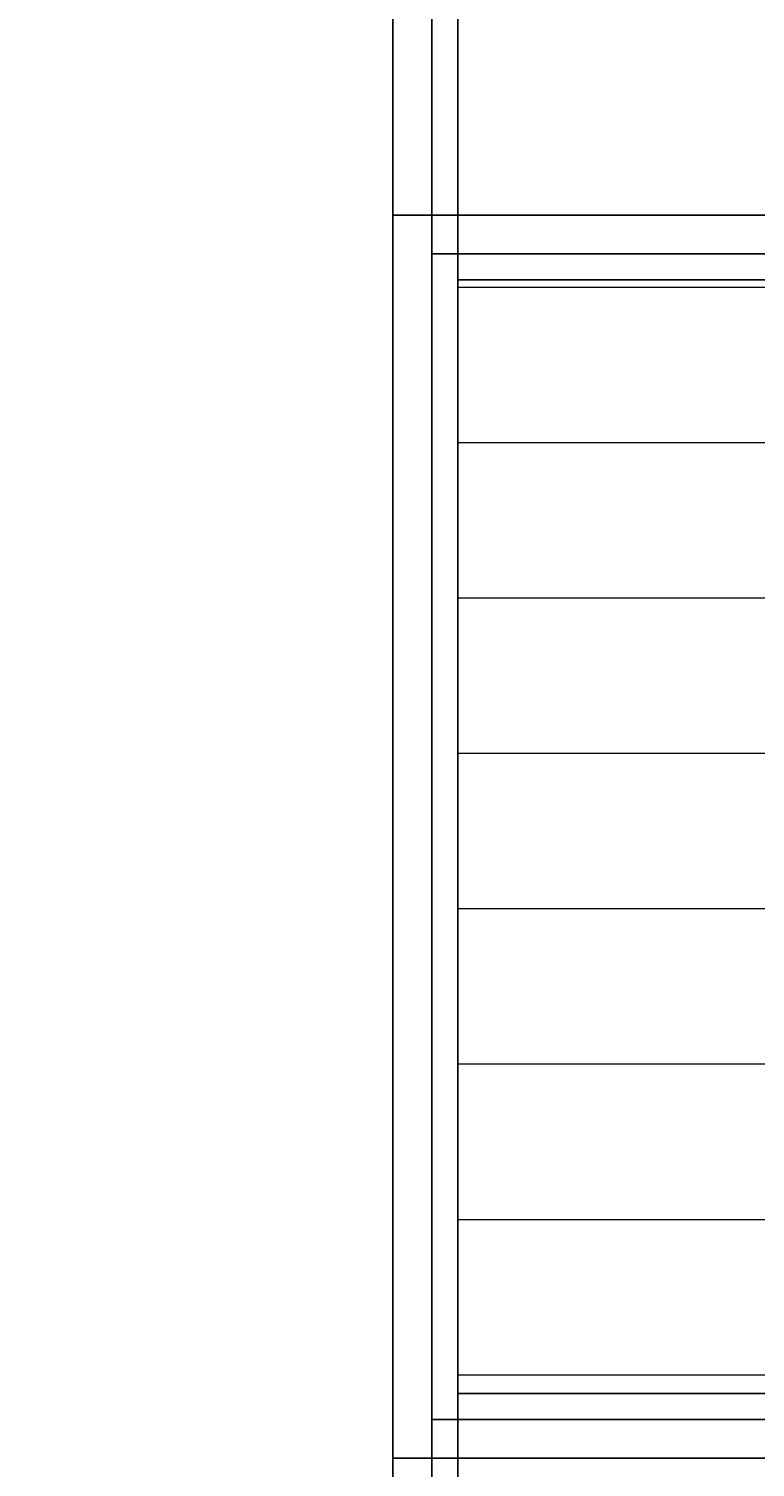
# Model space of a CAD drawing. Units: inches. Extents: x -6 to 289, y -8 to 323.
# Tile 37 of 107: x 174 to 202, y 68 to 124. Entities that reach past the tile are written whole.
import ezdxf

# ---------------------------------------------------------------- set-up
doc = ezdxf.new("R2010")
doc.units = ezdxf.units.IN
doc.header["$MEASUREMENT"] = 0
for name, color, linetype, lineweight in [('A-ANNO-DIMS', 2, 'Continuous', 18), ('A-ELEV-PATT', 8, 'Continuous', 13), ('A-GLAZ', 4, 'Continuous', 25)]:
    doc.layers.add(name, color=color, linetype=linetype, lineweight=lineweight)
doc.styles.get("Standard").update_dxf_attribs({"font": 'arial.ttf'})
doc.dimstyles.get("Standard").update_dxf_attribs({"dimtxt": 0.18, "dimasz": 0.18, "dimexe": 0.18, "dimexo": 0.0625, "dimgap": 0.09, "dimtad": 0, "dimtih": 1, "dimtoh": 1, "dimdec": 4, "dimzin": 0, "dimdsep": 46, "dimtxsty": 'Standard', "dimcen": 0.09, "dimadec": 0, "dimazin": 0, "dimtfac": 1, "dimtdec": 4, "dimtofl": 0, "dimtmove": 0, "dimatfit": 3, "dimfxl": 1, "dimtolj": 1, "dimtzin": 0, "dimarcsym": 0})

# ---------------------------------------------------------------- blocks, each defined once
blk = doc.blocks.new('*U4')
for p, q in [((1.5, 1.5), (1.5, 46.5)), ((1.5, 46.5), (21, 46.5)), ((21, 1.5), (21, 46.5)), ((21, 46.5), (40.5, 46.5)), ((40.5, 46.5), (40.5, 1.5)), ((21, 1.5), (1.5, 1.5)), ((40.5, 1.5), (21, 1.5))]:
    blk.add_line(p, q)
blk.add_lwpolyline([(0, 0), (0, 48), (42, 48), (42, 0)], close=True)
for points in [[(20, 45.5), (20, 2.5), (2.5, 2.5), (2.5, 45.5), (20, 45.5)], [(21, 45.5), (39.5, 45.5), (39.5, 2.5), (21, 2.5)]]:
    blk.add_lwpolyline(points)
blk = doc.blocks.new('*D40')
at = {"layer": 'A-ANNO-DIMS', "color": 0, "lineweight": -2, "transparency": 16777216}
for p, q in [((188.292, 226.826), (188.292, -8.391)), ((189.792, 225.326), (189.792, -8.391)), ((188.472, -8.211), (188.796, -8.211)), ((189.612, -8.211), (189.288, -8.211))]:
    blk.add_line(p, q, dxfattribs=at)
at = {"layer": 'A-ANNO-DIMS', "color": 0, "transparency": 16777216}
for points in [[(188.472, -8.181), (188.472, -8.241), (188.292, -8.211)], [(189.612, -8.181), (189.612, -8.241), (189.792, -8.211)]]:
    blk.add_solid(points, dxfattribs=at)
at = {"layer": 'Defpoints', "color": 0, "transparency": 16777216}
for p in [(188.292, 226.889), (189.792, 225.389), (189.792, -8.211)]:
    blk.add_point(p, dxfattribs=at)
at = {"layer": 'A-ANNO-DIMS', "color": 0, "transparency": 16777216, "insert": (189.042, -8.211), "char_height": 0.18, "attachment_point": 5}
blk.add_mtext('\\A1;1.5', dxfattribs=at)
blk = doc.blocks.new('*D41')
at = {"layer": 'A-ANNO-DIMS', "color": 0, "lineweight": -2, "transparency": 16777216}
for p, q in [((189.792, 225.326), (189.792, -8.391)), ((190.792, 224.326), (190.792, -8.391)), ((189.972, -8.211), (190.169, -8.211)), ((190.612, -8.211), (190.415, -8.211))]:
    blk.add_line(p, q, dxfattribs=at)
at = {"layer": 'A-ANNO-DIMS', "color": 0, "transparency": 16777216}
for points in [[(189.972, -8.181), (189.972, -8.241), (189.792, -8.211)], [(190.612, -8.181), (190.612, -8.241), (190.792, -8.211)]]:
    blk.add_solid(points, dxfattribs=at)
at = {"layer": 'Defpoints', "color": 0, "transparency": 16777216}
for p in [(189.792, 225.389), (190.792, 224.389), (190.792, -8.211)]:
    blk.add_point(p, dxfattribs=at)
at = {"layer": 'A-ANNO-DIMS', "color": 0, "transparency": 16777216, "insert": (190.292, -8.211), "char_height": 0.18, "attachment_point": 5}
blk.add_mtext('\\A1;1', dxfattribs=at)
blk = doc.blocks.new('*D42')
at = {"layer": 'A-ANNO-DIMS', "color": 0, "lineweight": -2, "transparency": 16777216}
for p, q in [((190.792, 224.326), (190.792, -8.391)), ((211.292, 224.326), (211.292, -8.391)), ((190.972, -8.211), (200.716, -8.211)), ((211.112, -8.211), (201.368, -8.211))]:
    blk.add_line(p, q, dxfattribs=at)
at = {"layer": 'A-ANNO-DIMS', "color": 0, "transparency": 16777216}
for points in [[(190.972, -8.181), (190.972, -8.241), (190.792, -8.211)], [(211.112, -8.181), (211.112, -8.241), (211.292, -8.211)]]:
    blk.add_solid(points, dxfattribs=at)
at = {"layer": 'Defpoints', "color": 0, "transparency": 16777216}
for p in [(190.792, 224.389), (211.292, 224.389), (211.292, -8.211)]:
    blk.add_point(p, dxfattribs=at)
at = {"layer": 'A-ANNO-DIMS', "color": 0, "transparency": 16777216, "insert": (201.042, -8.211), "char_height": 0.18, "attachment_point": 5}
blk.add_mtext('\\A1;20.5', dxfattribs=at)
blk = doc.blocks.new('*D79')
at = {"layer": 'A-ANNO-DIMS', "color": 0, "lineweight": -2, "transparency": 16777216}
for p, q in [((171.296, 118.033), (171.296, 322.969)), ((171.476, 322.789), (179.339, 322.789)), ((188.112, 322.789), (180.249, 322.789)), ((188.292, 116.842), (188.292, 322.969))]:
    blk.add_line(p, q, dxfattribs=at)
at = {"layer": 'A-ANNO-DIMS', "color": 0, "transparency": 16777216}
for points in [[(171.476, 322.819), (171.476, 322.759), (171.296, 322.789)], [(188.112, 322.819), (188.112, 322.759), (188.292, 322.789)]]:
    blk.add_solid(points, dxfattribs=at)
at = {"layer": 'Defpoints', "color": 0, "transparency": 16777216}
for p in [(188.292, 322.789), (171.296, 117.971), (188.292, 116.779)]:
    blk.add_point(p, dxfattribs=at)
at = {"layer": 'A-ANNO-DIMS', "color": 0, "transparency": 16777216, "insert": (179.794, 322.789), "char_height": 0.18, "attachment_point": 5}
blk.add_mtext('\\A1;16.996', dxfattribs=at)
blk = doc.blocks.new('*D80')
at = {"layer": 'A-ANNO-DIMS', "color": 0, "lineweight": -2, "transparency": 16777216}
for p, q in [((188.292, 116.842), (188.292, 322.969)), ((188.472, 322.789), (209.07, 322.789)), ((230.112, 322.789), (209.513, 322.789)), ((230.292, 116.842), (230.292, 322.969))]:
    blk.add_line(p, q, dxfattribs=at)
at = {"layer": 'A-ANNO-DIMS', "color": 0, "transparency": 16777216}
for points in [[(188.472, 322.819), (188.472, 322.759), (188.292, 322.789)], [(230.112, 322.819), (230.112, 322.759), (230.292, 322.789)]]:
    blk.add_solid(points, dxfattribs=at)
at = {"layer": 'Defpoints', "color": 0, "transparency": 16777216}
for p in [(230.292, 322.789), (188.292, 116.779), (230.292, 116.779)]:
    blk.add_point(p, dxfattribs=at)
at = {"layer": 'A-ANNO-DIMS', "color": 0, "transparency": 16777216, "insert": (209.292, 322.789), "char_height": 0.18, "attachment_point": 5}
blk.add_mtext('\\A1;42', dxfattribs=at)

msp = doc.modelspace()

# ---------------------------------------------------------------- hatches: boundary and pattern name
at = {"layer": 'A-ELEV-PATT'}
h = msp.add_hatch(dxfattribs=at)
h.set_pattern_fill('_USER', color=256, scale=6, pattern_type=0)
h.set_pattern_definition([(0, (0, 0), (0, 6), [])])
h.paths.add_polyline_path([(184.1244, 48.0851), (124.008, 48.0851), (124.008, 10.2888), (184.1244, 10.2888)])
h.paths.add_polyline_path([(244.2408, 48.0851), (186.3604, 48.0851), (186.3604, 10.2888), (244.2408, 10.2888)])
h.paths.add_polyline_path([(208.2918, 114.2795), (190.7918, 114.2795), (190.7918, 71.2795), (208.2918, 71.2795)])
h.paths.add_polyline_path([(227.7918, 114.2795), (209.2918, 114.2795), (209.2918, 71.2795), (227.7918, 71.2795)])
h.paths.add_polyline_path([(211.2918, 224.3887), (190.7918, 224.3887), (190.7918, 162.3484), (211.2918, 162.3484)])
h.paths.add_polyline_path([(233.7918, 224.3887), (212.2918, 224.3887), (212.2918, 162.3484), (233.7918, 162.3484)])
h.paths.add_polyline_path([(166.3835, 224.154), (147.8835, 224.154), (147.8835, 181.154), (166.3835, 181.154)])
h.paths.add_polyline_path([(146.8835, 224.154), (129.3835, 224.154), (129.3835, 181.154), (146.8835, 181.154)])

# ---------------------------------------------------------------- block references
at = {"layer": 'A-GLAZ'}
msp.add_blockref('*U4', (188.2918, 68.7795), dxfattribs=at)

# ---------------------------------------------------------------- dimensions: what is measured, and where the dimension line sits
at = {"layer": 'A-ANNO-DIMS'}
for base, p1, p2, override, picture, middle in [((188.2918, 322.7888), (171.296, 117.9706), (188.2918, 116.7795), {"dimdec": 3, "dimlfac": 1, "dimrnd": 0, "dimzin": 0, "dimdsep": 46, "dimlunit": 2}, '*D79', (179.7939, 322.7888)), ((230.2918, 322.7888), (188.2918, 116.7795), (230.2918, 116.7795), {"dimdec": 0, "dimlfac": 1, "dimrnd": 0, "dimzin": 0, "dimdsep": 46, "dimlunit": 2}, '*D80', (209.2918, 322.7888)), ((189.7918, -8.2112), (188.2918, 226.8887), (189.7918, 225.3887), {"dimdec": 1, "dimlfac": 1, "dimrnd": 0, "dimzin": 0, "dimdsep": 46, "dimlunit": 2}, '*D40', (189.0418, -8.2112)), ((190.7918, -8.2112), (189.7918, 225.3887), (190.7918, 224.3887), {"dimdec": 0, "dimlfac": 1, "dimrnd": 0, "dimzin": 0, "dimdsep": 46, "dimlunit": 2}, '*D41', (190.2918, -8.2112)), ((211.2918, -8.2112), (190.7918, 224.3887), (211.2918, 224.3887), {"dimdec": 1, "dimlfac": 1, "dimrnd": 0, "dimzin": 0, "dimdsep": 46, "dimlunit": 2}, '*D42', (201.0418, -8.2112))]:
    dim = msp.add_linear_dim(base=base, p1=p1, p2=p2, dimstyle='Standard', override=override, dxfattribs=at)
    dim.commit()
    dim.dimension.update_dxf_attribs({"geometry": picture, "text_midpoint": middle})

doc.saveas('drawing.dxf')
